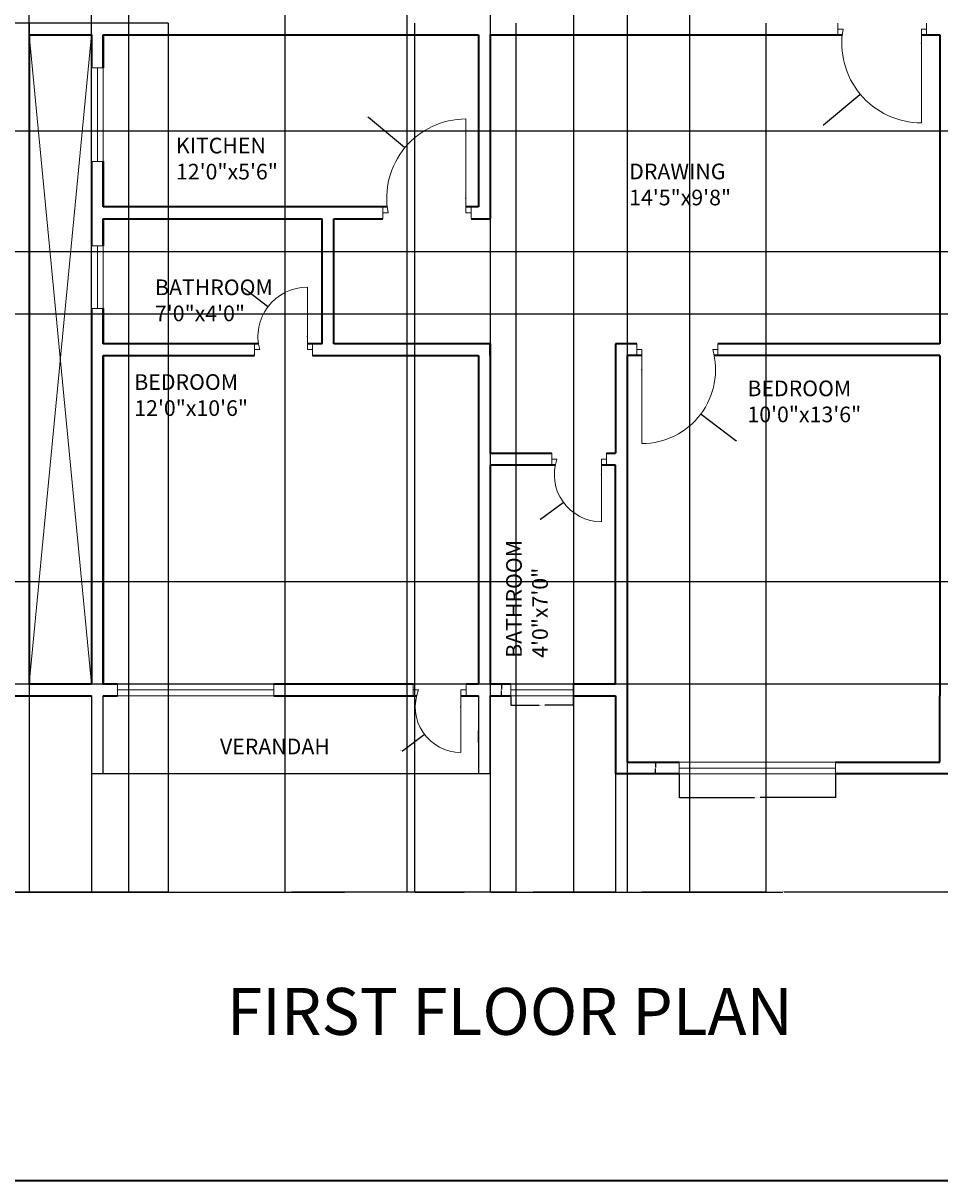
# Model space of a CAD drawing. Units: inches. Extents: x 1831 to 2867, y 1605 to 2524.
# Tile 2 of 7: x 2170 to 2522, y 1605 to 2049. Entities that reach past the tile are written whole.
import ezdxf

# ---------------------------------------------------------------- set-up
doc = ezdxf.new("R2010")
doc.units = ezdxf.units.IN
for name, color, linetype, lineweight in [('A-ANNO-DIMS', 2, 'Continuous', 18), ('A-ANNO-TEXT', 7, 'Continuous', 35), ('A-ANNO-TTLB', 7, 'Continuous', 35), ('A-AREA-IDEN', 7, 'Continuous', 18), ('A-DOOR', 11, 'Continuous', 18), ('A-FLOR-BALC', 7, 'Continuous', 25), ('A-FLOR-OPEN', 7, 'Continuous', 13), ('A-GLAZ', 121, 'Continuous', 18), ('A-WALL', 7, 'Continuous', 35)]:
    doc.layers.add(name, color=color, linetype=linetype, lineweight=lineweight)
doc.styles.get("Standard").update_dxf_attribs({"font": 'arial.ttf'})
doc.dimstyles.get("Standard").update_dxf_attribs({"dimtxt": 0.18, "dimasz": 0.18, "dimexe": 0.18, "dimexo": 0.0625, "dimgap": 0.09, "dimtad": 0, "dimtih": 1, "dimtoh": 1, "dimdec": 4, "dimzin": 0, "dimdsep": 46, "dimtxsty": 'Standard', "dimcen": 0.09, "dimadec": 0, "dimazin": 0, "dimtfac": 1, "dimtdec": 4, "dimtofl": 0, "dimtmove": 0, "dimatfit": 3, "dimfxl": 1, "dimtolj": 1, "dimtzin": 0, "dimarcsym": 0})

# ---------------------------------------------------------------- blocks, each defined once
blk = doc.blocks.new('WIN-60IN')
for p, q in [((4.5, 60), (0, 60)), ((0, 60), (2.25, 60)), ((0, 0), (0, 60)), ((2.25, 60), (2.25, 0)), ((4.5, 60), (4.5, 0)), ((4.5, 0), (0, 0)), ((2.25, 0), (4.5, 0))]:
    blk.add_line(p, q)
blk = doc.blocks.new('WIN-24IN')
for p, q in [((4.5, 24), (0, 24)), ((0, 24), (2.25, 24)), ((0, 0), (0, 24)), ((2.25, 24), (2.25, 0)), ((4.5, 0), (4.5, 24)), ((4.5, 0), (0, 0)), ((2.25, 0), (4.5, 0))]:
    blk.add_line(p, q)
blk = doc.blocks.new('WIN-36IN')
for p, q in [((0, 0), (0, 4.5)), ((36, 4.5), (0, 4.5)), ((36, 0), (36, 4.5)), ((36, 4.5), (36, 2.25)), ((36, 2.25), (0, 2.25)), ((0, 2.25), (0, 0)), ((0, 0), (36, 0))]:
    blk.add_line(p, q)
blk = doc.blocks.new('DOOR-LEAF-36IN')
for p, q in [((0, 2), (4.5, 2)), ((4.5, 2), (2.25, 2)), ((2.25, 2), (2.25, 0)), ((2.25, 0), (38.25, 0))]:
    blk.add_line(p, q)
blk = doc.blocks.new('DOOR-LEAF-36IN-ALT')
for p, q in [((36, 2), (0, 2)), ((33.75, 0), (38.25, 0)), ((36, 0), (36, 2)), ((38.25, 0), (36, 0))]:
    blk.add_line(p, q)
blk = doc.blocks.new('DOOR-LEAF-24IN')
for p, q in [((2.25, 0), (2.25, 2)), ((2.25, 2), (26.25, 2)), ((0, 0), (4.5, 0)), ((4.5, 0), (2.25, 0))]:
    blk.add_line(p, q)
blk = doc.blocks.new('DOOR-LEAF-24IN-ALT')
for p, q in [((24, 2), (0, 2)), ((21.75, 0), (26.25, 0)), ((24, 0), (24, 2)), ((26.25, 0), (24, 0))]:
    blk.add_line(p, q)
blk = doc.blocks.new('DOOR-STRIKE-JAMB')
for p, q in [((0, 0), (4.5, 0)), ((2.25, 0), (2.25, 2)), ((4.5, 0), (2.25, 0))]:
    blk.add_line(p, q)
blk = doc.blocks.new('*D16')
at = {"layer": 'A-ANNO-DIMS', "color": 0, "lineweight": -2, "transparency": 16777216}
for p, q in [((2356.89, 1791.11), (2356.89, 1787.39)), ((2380.89, 1791.11), (2380.89, 1787.39)), ((2357.07, 1787.57), (2367.77, 1787.57)), ((2380.71, 1787.57), (2370.01, 1787.57))]:
    blk.add_line(p, q, dxfattribs=at)
at = {"layer": 'A-ANNO-DIMS', "color": 0, "transparency": 16777216}
for points in [[(2357.07, 1787.6), (2357.07, 1787.54), (2356.89, 1787.57)], [(2380.71, 1787.6), (2380.71, 1787.54), (2380.89, 1787.57)]]:
    blk.add_solid(points, dxfattribs=at)
at = {"layer": 'Defpoints', "color": 0, "transparency": 16777216}
for p in [(2356.89, 1791.17), (2380.89, 1791.17), (2356.89, 1787.57)]:
    blk.add_point(p, dxfattribs=at)
at = {"layer": 'A-ANNO-DIMS', "color": 0, "transparency": 16777216, "insert": (2368.89, 1787.57), "char_height": 0.18, "attachment_point": 5}
blk.add_mtext('\\A1;WINDOW 24 TYP.', dxfattribs=at)
blk = doc.blocks.new('*D17')
at = {"layer": 'A-ANNO-DIMS', "color": 0, "lineweight": -2, "transparency": 16777216}
for p, q in [((2356.83, 1795.67), (2353.11, 1795.67)), ((2353.29, 1795.49), (2353.29, 1793.61)), ((2356.83, 1791.17), (2353.11, 1791.17)), ((2353.29, 1791.35), (2353.29, 1793.24))]:
    blk.add_line(p, q, dxfattribs=at)
at = {"layer": 'A-ANNO-DIMS', "color": 0, "transparency": 16777216}
for points in [[(2353.26, 1795.49), (2353.32, 1795.49), (2353.29, 1795.67)], [(2353.26, 1791.35), (2353.32, 1791.35), (2353.29, 1791.17)]]:
    blk.add_solid(points, dxfattribs=at)
at = {"layer": 'Defpoints', "color": 0, "transparency": 16777216}
for p in [(2353.29, 1795.67), (2356.89, 1795.67), (2356.89, 1791.17)]:
    blk.add_point(p, dxfattribs=at)
at = {"layer": 'A-ANNO-DIMS', "color": 0, "transparency": 16777216, "insert": (2353.29, 1793.42), "char_height": 0.18, "attachment_point": 5}
blk.add_mtext('\\A1;5 TYP.', dxfattribs=at)
blk = doc.blocks.new('*D20')
at = {"layer": 'A-ANNO-DIMS', "color": 0, "lineweight": -2, "transparency": 16777216}
for p, q in [((2421.49, 1761.11), (2421.49, 1751.99)), ((2481.49, 1761.11), (2481.49, 1751.99)), ((2421.67, 1752.17), (2450.37, 1752.17)), ((2481.31, 1752.17), (2452.61, 1752.17))]:
    blk.add_line(p, q, dxfattribs=at)
at = {"layer": 'A-ANNO-DIMS', "color": 0, "transparency": 16777216}
for points in [[(2421.67, 1752.2), (2421.67, 1752.14), (2421.49, 1752.17)], [(2481.31, 1752.2), (2481.31, 1752.14), (2481.49, 1752.17)]]:
    blk.add_solid(points, dxfattribs=at)
at = {"layer": 'Defpoints', "color": 0, "transparency": 16777216}
for p in [(2421.49, 1761.17), (2481.49, 1761.17), (2421.49, 1752.17)]:
    blk.add_point(p, dxfattribs=at)
at = {"layer": 'A-ANNO-DIMS', "color": 0, "transparency": 16777216, "insert": (2451.49, 1752.17), "char_height": 0.18, "attachment_point": 5}
blk.add_mtext('\\A1;WINDOW 60 TYP.', dxfattribs=at)
blk = doc.blocks.new('*D21')
at = {"layer": 'A-ANNO-DIMS', "color": 0, "lineweight": -2, "transparency": 16777216}
for p, q in [((2421.43, 1765.67), (2412.31, 1765.67)), ((2412.49, 1765.49), (2412.49, 1763.61)), ((2412.49, 1761.35), (2412.49, 1763.24)), ((2421.43, 1761.17), (2412.31, 1761.17))]:
    blk.add_line(p, q, dxfattribs=at)
at = {"layer": 'A-ANNO-DIMS', "color": 0, "transparency": 16777216}
for points in [[(2412.46, 1765.49), (2412.52, 1765.49), (2412.49, 1765.67)], [(2412.46, 1761.35), (2412.52, 1761.35), (2412.49, 1761.17)]]:
    blk.add_solid(points, dxfattribs=at)
at = {"layer": 'Defpoints', "color": 0, "transparency": 16777216}
for p in [(2412.49, 1765.67), (2421.49, 1765.67), (2421.49, 1761.17)]:
    blk.add_point(p, dxfattribs=at)
at = {"layer": 'A-ANNO-DIMS', "color": 0, "transparency": 16777216, "insert": (2412.49, 1763.42), "char_height": 0.18, "attachment_point": 5}
blk.add_mtext('\\A1;5 TYP.', dxfattribs=at)
blk = doc.blocks.new('*D25')
at = {"layer": 'A-ANNO-DIMS', "color": 0, "lineweight": -2, "transparency": 16777216}
for p, q in [((2055.05, 1761.11), (2055.05, 1715.69)), ((2196.05, 1761.11), (2196.05, 1715.69)), ((2055.23, 1715.87), (2125.29, 1715.87)), ((2195.87, 1715.87), (2125.81, 1715.87))]:
    blk.add_line(p, q, dxfattribs=at)
at = {"layer": 'A-ANNO-DIMS', "color": 0, "transparency": 16777216}
for points in [[(2055.23, 1715.9), (2055.23, 1715.84), (2055.05, 1715.87)], [(2195.87, 1715.9), (2195.87, 1715.84), (2196.05, 1715.87)]]:
    blk.add_solid(points, dxfattribs=at)
at = {"layer": 'Defpoints', "color": 0, "transparency": 16777216}
for p in [(2055.05, 1761.17), (2196.05, 1761.17), (2196.05, 1715.87)]:
    blk.add_point(p, dxfattribs=at)
at = {"layer": 'A-ANNO-DIMS', "color": 0, "transparency": 16777216, "insert": (2125.55, 1715.87), "char_height": 0.18, "attachment_point": 5}
blk.add_mtext('\\A1;141', dxfattribs=at)
blk = doc.blocks.new('*D26')
at = {"layer": 'A-ANNO-DIMS', "color": 0, "lineweight": -2, "transparency": 16777216}
for p, q in [((2196.05, 1761.11), (2196.05, 1715.69)), ((2349.05, 1761.11), (2349.05, 1715.69)), ((2196.23, 1715.87), (2272.27, 1715.87)), ((2348.87, 1715.87), (2272.83, 1715.87))]:
    blk.add_line(p, q, dxfattribs=at)
at = {"layer": 'A-ANNO-DIMS', "color": 0, "transparency": 16777216}
for points in [[(2196.23, 1715.9), (2196.23, 1715.84), (2196.05, 1715.87)], [(2348.87, 1715.9), (2348.87, 1715.84), (2349.05, 1715.87)]]:
    blk.add_solid(points, dxfattribs=at)
at = {"layer": 'Defpoints', "color": 0, "transparency": 16777216}
for p in [(2196.05, 1761.17), (2349.05, 1761.17), (2349.05, 1715.87)]:
    blk.add_point(p, dxfattribs=at)
at = {"layer": 'A-ANNO-DIMS', "color": 0, "transparency": 16777216, "insert": (2272.55, 1715.87), "char_height": 0.18, "attachment_point": 5}
blk.add_mtext('\\A1;153', dxfattribs=at)
blk = doc.blocks.new('*D27')
at = {"layer": 'A-ANNO-DIMS', "color": 0, "lineweight": -2, "transparency": 16777216}
for p, q in [((2349.05, 1761.11), (2349.05, 1715.69)), ((2397.05, 1761.11), (2397.05, 1715.69)), ((2349.23, 1715.87), (2372.83, 1715.87)), ((2396.87, 1715.87), (2373.27, 1715.87))]:
    blk.add_line(p, q, dxfattribs=at)
at = {"layer": 'A-ANNO-DIMS', "color": 0, "transparency": 16777216}
for points in [[(2349.23, 1715.9), (2349.23, 1715.84), (2349.05, 1715.87)], [(2396.87, 1715.9), (2396.87, 1715.84), (2397.05, 1715.87)]]:
    blk.add_solid(points, dxfattribs=at)
at = {"layer": 'Defpoints', "color": 0, "transparency": 16777216}
for p in [(2349.05, 1761.17), (2397.05, 1761.17), (2397.05, 1715.87)]:
    blk.add_point(p, dxfattribs=at)
at = {"layer": 'A-ANNO-DIMS', "color": 0, "transparency": 16777216, "insert": (2373.05, 1715.87), "char_height": 0.18, "attachment_point": 5}
blk.add_mtext('\\A1;48', dxfattribs=at)
blk = doc.blocks.new('*D28')
at = {"layer": 'A-ANNO-DIMS', "color": 0, "lineweight": -2, "transparency": 16777216}
for p, q in [((2397.05, 1761.11), (2397.05, 1715.69)), ((2526.05, 1761.11), (2526.05, 1715.69)), ((2397.23, 1715.87), (2461.27, 1715.87)), ((2525.87, 1715.87), (2461.83, 1715.87))]:
    blk.add_line(p, q, dxfattribs=at)
at = {"layer": 'A-ANNO-DIMS', "color": 0, "transparency": 16777216}
for points in [[(2397.23, 1715.9), (2397.23, 1715.84), (2397.05, 1715.87)], [(2525.87, 1715.9), (2525.87, 1715.84), (2526.05, 1715.87)]]:
    blk.add_solid(points, dxfattribs=at)
at = {"layer": 'Defpoints', "color": 0, "transparency": 16777216}
for p in [(2397.05, 1761.17), (2526.05, 1761.17), (2526.05, 1715.87)]:
    blk.add_point(p, dxfattribs=at)
at = {"layer": 'A-ANNO-DIMS', "color": 0, "transparency": 16777216, "insert": (2461.55, 1715.87), "char_height": 0.18, "attachment_point": 5}
blk.add_mtext('\\A1;129', dxfattribs=at)
blk = doc.blocks.new('*D41')
at = {"layer": 'A-ANNO-DIMS', "color": 0, "lineweight": -2, "transparency": 16777216}
for p, q in [((2156.64, 2387.11), (2156.64, 1715.69)), ((2210.17, 2387.11), (2210.17, 1715.69)), ((2156.82, 1715.87), (2183.01, 1715.87)), ((2209.99, 1715.87), (2183.8, 1715.87))]:
    blk.add_line(p, q, dxfattribs=at)
at = {"layer": 'A-ANNO-DIMS', "color": 0, "transparency": 16777216}
for points in [[(2156.82, 1715.9), (2156.82, 1715.84), (2156.64, 1715.87)], [(2209.99, 1715.9), (2209.99, 1715.84), (2210.17, 1715.87)]]:
    blk.add_solid(points, dxfattribs=at)
at = {"layer": 'Defpoints', "color": 0, "transparency": 16777216}
for p in [(2156.64, 2387.17), (2210.17, 2387.17), (2210.17, 1715.87)]:
    blk.add_point(p, dxfattribs=at)
at = {"layer": 'A-ANNO-DIMS', "color": 0, "transparency": 16777216, "insert": (2183.4, 1715.87), "char_height": 0.18, "attachment_point": 5}
blk.add_mtext('\\A1;53.52', dxfattribs=at)
blk = doc.blocks.new('*D42')
at = {"layer": 'A-ANNO-DIMS', "color": 0, "lineweight": -2, "transparency": 16777216}
for p, q in [((2270.17, 2391.61), (2270.17, 1715.69)), ((2316.97, 2391.61), (2316.97, 1715.69)), ((2270.35, 1715.87), (2293.1, 1715.87)), ((2316.79, 1715.87), (2294.04, 1715.87))]:
    blk.add_line(p, q, dxfattribs=at)
at = {"layer": 'A-ANNO-DIMS', "color": 0, "transparency": 16777216}
for points in [[(2270.35, 1715.9), (2270.35, 1715.84), (2270.17, 1715.87)], [(2316.79, 1715.9), (2316.79, 1715.84), (2316.97, 1715.87)]]:
    blk.add_solid(points, dxfattribs=at)
at = {"layer": 'Defpoints', "color": 0, "transparency": 16777216}
for p in [(2270.17, 2391.67), (2316.97, 2391.67), (2316.97, 1715.87)]:
    blk.add_point(p, dxfattribs=at)
at = {"layer": 'A-ANNO-DIMS', "color": 0, "transparency": 16777216, "insert": (2293.57, 1715.87), "char_height": 0.18, "attachment_point": 5}
blk.add_mtext('\\A1;46.805', dxfattribs=at)
blk = doc.blocks.new('*D43')
at = {"layer": 'A-ANNO-DIMS', "color": 0, "lineweight": -2, "transparency": 16777216}
for p, q in [((2349.05, 2387.11), (2349.05, 1715.69)), ((2381.01, 2387.11), (2381.01, 1715.69)), ((2349.23, 1715.87), (2364.57, 1715.87)), ((2380.83, 1715.87), (2365.49, 1715.87))]:
    blk.add_line(p, q, dxfattribs=at)
at = {"layer": 'A-ANNO-DIMS', "color": 0, "transparency": 16777216}
for points in [[(2349.23, 1715.9), (2349.23, 1715.84), (2349.05, 1715.87)], [(2380.83, 1715.9), (2380.83, 1715.84), (2381.01, 1715.87)]]:
    blk.add_solid(points, dxfattribs=at)
at = {"layer": 'Defpoints', "color": 0, "transparency": 16777216}
for p in [(2349.05, 2387.17), (2381.01, 2387.17), (2381.01, 1715.87)]:
    blk.add_point(p, dxfattribs=at)
at = {"layer": 'A-ANNO-DIMS', "color": 0, "transparency": 16777216, "insert": (2365.03, 1715.87), "char_height": 0.18, "attachment_point": 5}
blk.add_mtext('\\A1;31.956', dxfattribs=at)
blk = doc.blocks.new('*D44')
at = {"layer": 'A-ANNO-DIMS', "color": 0, "lineweight": -2, "transparency": 16777216}
for p, q in [((2401.55, 2417.11), (2401.55, 1715.69)), ((2425.47, 2417.11), (2425.47, 1715.69)), ((2401.73, 1715.87), (2413.05, 1715.87)), ((2425.29, 1715.87), (2413.98, 1715.87))]:
    blk.add_line(p, q, dxfattribs=at)
at = {"layer": 'A-ANNO-DIMS', "color": 0, "transparency": 16777216}
for points in [[(2401.73, 1715.9), (2401.73, 1715.84), (2401.55, 1715.87)], [(2425.29, 1715.9), (2425.29, 1715.84), (2425.47, 1715.87)]]:
    blk.add_solid(points, dxfattribs=at)
at = {"layer": 'Defpoints', "color": 0, "transparency": 16777216}
for p in [(2401.55, 2417.17), (2425.47, 2417.17), (2425.47, 1715.87)]:
    blk.add_point(p, dxfattribs=at)
at = {"layer": 'A-ANNO-DIMS', "color": 0, "transparency": 16777216, "insert": (2413.51, 1715.87), "char_height": 0.18, "attachment_point": 5}
blk.add_mtext('\\A1;23.924', dxfattribs=at)
blk = doc.blocks.new('*D53')
at = {"layer": 'A-ANNO-DIMS', "color": 0, "lineweight": -2, "transparency": 16777216}
for p, q in [((2786.99, 2007.7), (1844.57, 2007.7)), ((1844.75, 2007.52), (1844.75, 1984.78)), ((1844.75, 1961.67), (1844.75, 1984.41)), ((2786.99, 1961.49), (1844.57, 1961.49))]:
    blk.add_line(p, q, dxfattribs=at)
at = {"layer": 'A-ANNO-DIMS', "color": 0, "transparency": 16777216}
for points in [[(1844.72, 2007.52), (1844.78, 2007.52), (1844.75, 2007.7)], [(1844.72, 1961.67), (1844.78, 1961.67), (1844.75, 1961.49)]]:
    blk.add_solid(points, dxfattribs=at)
at = {"layer": 'Defpoints', "color": 0, "transparency": 16777216}
for p in [(2787.05, 2007.7), (1844.75, 1961.49), (2787.05, 1961.49)]:
    blk.add_point(p, dxfattribs=at)
at = {"layer": 'A-ANNO-DIMS', "color": 0, "transparency": 16777216, "insert": (1844.75, 1984.59), "char_height": 0.18, "attachment_point": 5}
blk.add_mtext('\\A1;46.2', dxfattribs=at)
blk = doc.blocks.new('*D54')
at = {"layer": 'A-ANNO-DIMS', "color": 0, "lineweight": -2, "transparency": 16777216}
for p, q in [((2786.99, 1937.49), (1844.57, 1937.49)), ((1844.75, 1937.31), (1844.75, 1886.37)), ((1844.75, 1835.06), (1844.75, 1886)), ((2786.99, 1834.88), (1844.57, 1834.88))]:
    blk.add_line(p, q, dxfattribs=at)
at = {"layer": 'A-ANNO-DIMS', "color": 0, "transparency": 16777216}
for points in [[(1844.72, 1937.31), (1844.78, 1937.31), (1844.75, 1937.49)], [(1844.72, 1835.06), (1844.78, 1835.06), (1844.75, 1834.88)]]:
    blk.add_solid(points, dxfattribs=at)
at = {"layer": 'Defpoints', "color": 0, "transparency": 16777216}
for p in [(2787.05, 1937.49), (1844.75, 1834.88), (2787.05, 1834.88)]:
    blk.add_point(p, dxfattribs=at)
at = {"layer": 'A-ANNO-DIMS', "color": 0, "transparency": 16777216, "insert": (1844.75, 1886.19), "char_height": 0.18, "attachment_point": 5}
blk.add_mtext('\\A1;102.61', dxfattribs=at)
blk = doc.blocks.new('*D55')
at = {"layer": 'A-ANNO-DIMS', "color": 0, "lineweight": -2, "transparency": 16777216}
for p, q in [((2786.99, 1834.88), (1844.57, 1834.88)), ((1844.75, 1834.7), (1844.75, 1815.46)), ((1844.75, 1795.85), (1844.75, 1815.09)), ((2786.99, 1795.67), (1844.57, 1795.67))]:
    blk.add_line(p, q, dxfattribs=at)
at = {"layer": 'A-ANNO-DIMS', "color": 0, "transparency": 16777216}
for points in [[(1844.72, 1834.7), (1844.78, 1834.7), (1844.75, 1834.88)], [(1844.72, 1795.85), (1844.78, 1795.85), (1844.75, 1795.67)]]:
    blk.add_solid(points, dxfattribs=at)
at = {"layer": 'Defpoints', "color": 0, "transparency": 16777216}
for p in [(2787.05, 1834.88), (1844.75, 1795.67), (2787.05, 1795.67)]:
    blk.add_point(p, dxfattribs=at)
at = {"layer": 'A-ANNO-DIMS', "color": 0, "transparency": 16777216, "insert": (1844.75, 1815.28), "char_height": 0.18, "attachment_point": 5}
blk.add_mtext('\\A1;39.206', dxfattribs=at)
blk = doc.blocks.new('*D56')
at = {"layer": 'A-ANNO-DIMS', "color": 0, "lineweight": -2, "transparency": 16777216}
for p, q in [((2172.05, 2049.11), (2172.05, 1715.69)), ((2225.49, 2049.11), (2225.49, 1715.69)), ((2172.23, 1715.87), (2198.38, 1715.87)), ((2225.31, 1715.87), (2199.17, 1715.87))]:
    blk.add_line(p, q, dxfattribs=at)
at = {"layer": 'A-ANNO-DIMS', "color": 0, "transparency": 16777216}
for points in [[(2172.23, 1715.9), (2172.23, 1715.84), (2172.05, 1715.87)], [(2225.31, 1715.9), (2225.31, 1715.84), (2225.49, 1715.87)]]:
    blk.add_solid(points, dxfattribs=at)
at = {"layer": 'Defpoints', "color": 0, "transparency": 16777216}
for p in [(2172.05, 2049.17), (2225.49, 2049.17), (2225.49, 1715.87)]:
    blk.add_point(p, dxfattribs=at)
at = {"layer": 'A-ANNO-DIMS', "color": 0, "transparency": 16777216, "insert": (2198.77, 1715.87), "char_height": 0.18, "attachment_point": 5}
blk.add_mtext('\\A1;53.44', dxfattribs=at)
blk = doc.blocks.new('*D57')
at = {"layer": 'A-ANNO-DIMS', "color": 0, "lineweight": -2, "transparency": 16777216}
for p, q in [((2225.49, 2049.11), (2225.49, 1715.69)), ((2319.99, 2049.11), (2319.99, 1715.69)), ((2225.67, 1715.87), (2272.42, 1715.87)), ((2319.81, 1715.87), (2273.06, 1715.87))]:
    blk.add_line(p, q, dxfattribs=at)
at = {"layer": 'A-ANNO-DIMS', "color": 0, "transparency": 16777216}
for points in [[(2225.67, 1715.9), (2225.67, 1715.84), (2225.49, 1715.87)], [(2319.81, 1715.9), (2319.81, 1715.84), (2319.99, 1715.87)]]:
    blk.add_solid(points, dxfattribs=at)
at = {"layer": 'Defpoints', "color": 0, "transparency": 16777216}
for p in [(2225.49, 2049.17), (2319.99, 2049.17), (2319.99, 1715.87)]:
    blk.add_point(p, dxfattribs=at)
at = {"layer": 'A-ANNO-DIMS', "color": 0, "transparency": 16777216, "insert": (2272.74, 1715.87), "char_height": 0.18, "attachment_point": 5}
blk.add_mtext('\\A1;94.5', dxfattribs=at)
blk = doc.blocks.new('*D58')
at = {"layer": 'A-ANNO-DIMS', "color": 0, "lineweight": -2, "transparency": 16777216}
for p, q in [((2319.99, 2049.11), (2319.99, 1715.69)), ((2358.81, 2049.11), (2358.81, 1715.69)), ((2320.17, 1715.87), (2339, 1715.87)), ((2358.63, 1715.87), (2339.79, 1715.87))]:
    blk.add_line(p, q, dxfattribs=at)
at = {"layer": 'A-ANNO-DIMS', "color": 0, "transparency": 16777216}
for points in [[(2320.17, 1715.9), (2320.17, 1715.84), (2319.99, 1715.87)], [(2358.63, 1715.9), (2358.63, 1715.84), (2358.81, 1715.87)]]:
    blk.add_solid(points, dxfattribs=at)
at = {"layer": 'Defpoints', "color": 0, "transparency": 16777216}
for p in [(2319.99, 2049.17), (2358.81, 2049.17), (2358.81, 1715.87)]:
    blk.add_point(p, dxfattribs=at)
at = {"layer": 'A-ANNO-DIMS', "color": 0, "transparency": 16777216, "insert": (2339.4, 1715.87), "char_height": 0.18, "attachment_point": 5}
blk.add_mtext('\\A1;38.82', dxfattribs=at)
blk = doc.blocks.new('*D59')
at = {"layer": 'A-ANNO-DIMS', "color": 0, "lineweight": -2, "transparency": 16777216}
for p, q in [((2358.81, 2049.11), (2358.81, 1715.69)), ((2454.81, 2049.11), (2454.81, 1715.69)), ((2358.99, 1715.87), (2406.59, 1715.87)), ((2454.63, 1715.87), (2407.02, 1715.87))]:
    blk.add_line(p, q, dxfattribs=at)
at = {"layer": 'A-ANNO-DIMS', "color": 0, "transparency": 16777216}
for points in [[(2358.99, 1715.9), (2358.99, 1715.84), (2358.81, 1715.87)], [(2454.63, 1715.9), (2454.63, 1715.84), (2454.81, 1715.87)]]:
    blk.add_solid(points, dxfattribs=at)
at = {"layer": 'Defpoints', "color": 0, "transparency": 16777216}
for p in [(2358.81, 2049.17), (2454.81, 2049.17), (2454.81, 1715.87)]:
    blk.add_point(p, dxfattribs=at)
at = {"layer": 'A-ANNO-DIMS', "color": 0, "transparency": 16777216, "insert": (2406.81, 1715.87), "char_height": 0.18, "attachment_point": 5}
blk.add_mtext('\\A1;96', dxfattribs=at)
blk = doc.blocks.new('*D60')
at = {"layer": 'A-ANNO-DIMS', "color": 0, "lineweight": -2, "transparency": 16777216}
for p, q in [((2225.43, 2091.42), (1844.57, 2091.42)), ((1844.75, 2091.24), (1844.75, 2070.48)), ((1844.75, 2049.35), (1844.75, 2070.12)), ((2225.43, 2049.17), (1844.57, 2049.17))]:
    blk.add_line(p, q, dxfattribs=at)
at = {"layer": 'A-ANNO-DIMS', "color": 0, "transparency": 16777216}
for points in [[(1844.72, 2091.24), (1844.78, 2091.24), (1844.75, 2091.42)], [(1844.72, 2049.35), (1844.78, 2049.35), (1844.75, 2049.17)]]:
    blk.add_solid(points, dxfattribs=at)
at = {"layer": 'Defpoints', "color": 0, "transparency": 16777216}
for p in [(1844.75, 2091.42), (2225.49, 2091.42), (2225.49, 2049.17)]:
    blk.add_point(p, dxfattribs=at)
at = {"layer": 'A-ANNO-DIMS', "color": 0, "transparency": 16777216, "insert": (1844.75, 2070.3), "char_height": 0.18, "attachment_point": 5}
blk.add_mtext('\\A1;42.25', dxfattribs=at)
blk = doc.blocks.new('*D63')
at = {"layer": 'A-ANNO-DIMS', "color": 0, "lineweight": -2, "transparency": 16777216}
for p, q in [((2172.05, 1795.74), (2172.05, 2467.15)), ((2172.23, 2466.97), (2183.83, 2466.97)), ((2195.87, 2466.97), (2184.27, 2466.97)), ((2196.05, 1795.74), (2196.05, 2467.15))]:
    blk.add_line(p, q, dxfattribs=at)
at = {"layer": 'A-ANNO-DIMS', "color": 0, "transparency": 16777216}
for points in [[(2172.23, 2467), (2172.23, 2466.94), (2172.05, 2466.97)], [(2195.87, 2467), (2195.87, 2466.94), (2196.05, 2466.97)]]:
    blk.add_solid(points, dxfattribs=at)
at = {"layer": 'Defpoints', "color": 0, "transparency": 16777216}
for p in [(2196.05, 2466.97), (2172.05, 1795.67), (2196.05, 1795.67)]:
    blk.add_point(p, dxfattribs=at)
at = {"layer": 'A-ANNO-DIMS', "color": 0, "transparency": 16777216, "insert": (2184.05, 2466.97), "char_height": 0.18, "attachment_point": 5}
blk.add_mtext('\\A1;24', dxfattribs=at)
blk = doc.blocks.new('*D66')
at = {"layer": 'A-ANNO-DIMS', "color": 0, "lineweight": -2, "transparency": 16777216}
for p, q in [((2514.4, 2041.48), (2514.58, 2041.48)), ((2514.49, 2041.39), (2514.49, 2041.57)), ((2476.96, 2010.14), (2490.9, 2021.78)), ((2476.78, 2010.14), (2476.96, 2010.14))]:
    blk.add_line(p, q, dxfattribs=at)
at = {"layer": 'A-ANNO-DIMS', "color": 0, "transparency": 16777216}
blk.add_solid([(2490.88, 2021.8), (2490.92, 2021.75), (2491.04, 2021.89)], dxfattribs=at)
at = {"layer": 'Defpoints', "color": 0, "transparency": 16777216}
for p in [(2514.49, 2041.48), (2491.04, 2021.89)]:
    blk.add_point(p, dxfattribs=at)
at = {"layer": 'A-ANNO-DIMS', "color": 0, "transparency": 16777216, "insert": (2476.3, 2010.14), "char_height": 0.18, "attachment_point": 5}
blk.add_mtext('\\A1;R30.56', dxfattribs=at)
blk = doc.blocks.new('*D67')
at = {"layer": 'A-ANNO-DIMS', "color": 0, "lineweight": -2, "transparency": 16777216}
for p, q in [((2302.1, 2013.08), (2302.28, 2013.08)), ((2302.28, 2013.08), (2316.18, 2001.55)), ((2339.62, 1982.03), (2339.8, 1982.03)), ((2339.71, 1981.94), (2339.71, 1982.12))]:
    blk.add_line(p, q, dxfattribs=at)
at = {"layer": 'A-ANNO-DIMS', "color": 0, "transparency": 16777216}
blk.add_solid([(2316.2, 2001.58), (2316.16, 2001.53), (2316.32, 2001.44)], dxfattribs=at)
at = {"layer": 'Defpoints', "color": 0, "transparency": 16777216}
for p in [(2316.32, 2001.44), (2339.71, 1982.03)]:
    blk.add_point(p, dxfattribs=at)
at = {"layer": 'A-ANNO-DIMS', "color": 0, "transparency": 16777216, "insert": (2301.55, 2013.08), "char_height": 0.18, "attachment_point": 5}
blk.add_mtext('\\A1;R30.395', dxfattribs=at)
blk = doc.blocks.new('*D71')
at = {"layer": 'A-ANNO-DIMS', "color": 0, "lineweight": -2, "transparency": 16777216}
for p, q in [((2407.14, 1916.17), (2407.32, 1916.17)), ((2407.23, 1916.08), (2407.23, 1916.26)), ((2443.31, 1888.95), (2429.92, 1899.05)), ((2443.49, 1888.95), (2443.31, 1888.95))]:
    blk.add_line(p, q, dxfattribs=at)
at = {"layer": 'A-ANNO-DIMS', "color": 0, "transparency": 16777216}
blk.add_solid([(2429.94, 1899.07), (2429.9, 1899.03), (2429.78, 1899.16)], dxfattribs=at)
at = {"layer": 'Defpoints', "color": 0, "transparency": 16777216}
for p in [(2407.23, 1916.17), (2429.78, 1899.16)]:
    blk.add_point(p, dxfattribs=at)
at = {"layer": 'A-ANNO-DIMS', "color": 0, "transparency": 16777216, "insert": (2443.97, 1888.95), "char_height": 0.18, "attachment_point": 5}
blk.add_mtext('\\A1;R28.25', dxfattribs=at)
blk = doc.blocks.new('*D90')
at = {"layer": 'A-ANNO-DIMS', "color": 0, "lineweight": -2, "transparency": 16777216}
for p, q in [((2254.54, 1947.34), (2254.72, 1947.34)), ((2254.72, 1947.34), (2263.62, 1940.56)), ((2278.76, 1928.97), (2278.94, 1928.97)), ((2278.85, 1928.88), (2278.85, 1929.06))]:
    blk.add_line(p, q, dxfattribs=at)
at = {"layer": 'A-ANNO-DIMS', "color": 0, "transparency": 16777216}
blk.add_solid([(2263.64, 1940.58), (2263.61, 1940.54), (2263.77, 1940.45)], dxfattribs=at)
at = {"layer": 'Defpoints', "color": 0, "transparency": 16777216}
for p in [(2263.77, 1940.45), (2278.85, 1928.97)]:
    blk.add_point(p, dxfattribs=at)
at = {"layer": 'A-ANNO-DIMS', "color": 0, "transparency": 16777216, "insert": (2253.99, 1947.34), "char_height": 0.18, "attachment_point": 5}
blk.add_mtext('\\A1;R18.956', dxfattribs=at)
blk = doc.blocks.new('*D98')
at = {"layer": 'A-ANNO-DIMS', "color": 0, "lineweight": -2, "transparency": 16777216}
for p, q in [((2391.61, 1876), (2391.79, 1876)), ((2391.7, 1875.91), (2391.7, 1876.09)), ((2368.34, 1858.95), (2376.95, 1865.24)), ((2368.16, 1858.95), (2368.34, 1858.95))]:
    blk.add_line(p, q, dxfattribs=at)
at = {"layer": 'A-ANNO-DIMS', "color": 0, "transparency": 16777216}
blk.add_solid([(2376.93, 1865.26), (2376.97, 1865.21), (2377.1, 1865.34)], dxfattribs=at)
at = {"layer": 'Defpoints', "color": 0, "transparency": 16777216}
for p in [(2391.7, 1876), (2377.1, 1865.34)]:
    blk.add_point(p, dxfattribs=at)
at = {"layer": 'A-ANNO-DIMS', "color": 0, "transparency": 16777216, "insert": (2367.61, 1858.95), "char_height": 0.18, "attachment_point": 5}
blk.add_mtext('\\A1;R18.077', dxfattribs=at)
blk = doc.blocks.new('*D101')
at = {"layer": 'A-ANNO-DIMS', "color": 0, "lineweight": -2, "transparency": 16777216}
for p, q in [((2337.64, 1786.9), (2337.82, 1786.9)), ((2337.73, 1786.81), (2337.73, 1786.99)), ((2315.4, 1770.07), (2323.63, 1776.27)), ((2315.22, 1770.07), (2315.4, 1770.07))]:
    blk.add_line(p, q, dxfattribs=at)
at = {"layer": 'A-ANNO-DIMS', "color": 0, "transparency": 16777216}
blk.add_solid([(2323.61, 1776.3), (2323.65, 1776.25), (2323.77, 1776.38)], dxfattribs=at)
at = {"layer": 'Defpoints', "color": 0, "transparency": 16777216}
for p in [(2337.73, 1786.9), (2323.77, 1776.38)]:
    blk.add_point(p, dxfattribs=at)
at = {"layer": 'A-ANNO-DIMS', "color": 0, "transparency": 16777216, "insert": (2314.74, 1770.07), "char_height": 0.18, "attachment_point": 5}
blk.add_mtext('\\A1;R17.48', dxfattribs=at)

msp = doc.modelspace()

# ---------------------------------------------------------------- linework, layer by layer
at = {"layer": 'A-ANNO-TTLB'}
msp.add_lwpolyline([(1831.1248, 2523.9204), (2867.0416, 2523.9204), (2867.0416, 1605.0781), (1831.1248, 1605.0781)], close=True, dxfattribs=at)
at = {"layer": 'A-DOOR'}
for centre, radius, start, end in [((2514.4879, 2041.481), 30.5572, 169.739837, 270), ((2339.7066, 1982.0286), 30.3952, 90, 190.626041), ((2278.8502, 1928.9679), 18.9559, 90, 195.432084), ((2407.228, 1916.1727), 28.2489, 270, 15.925435), ((2391.6972, 1876.0006), 18.0768, 160.872592, 270), ((2337.7334, 1786.9033), 17.4795, 158.097162, 270)]:
    msp.add_arc(centre, radius, start, end, dxfattribs=at)
at = {"layer": 'A-FLOR-BALC'}
for p, q in [((2196.051, 1791.1738), (2196.051, 1761.1738)), ((2200.551, 1761.1738), (2200.551, 1791.1738)), ((2344.551, 1791.1738), (2344.551, 1761.1738)), ((2349.051, 1761.1738), (2349.051, 1791.1738)), ((2344.551, 1773.1738), (2344.551, 1777.6738)), ((2349.051, 1761.1738), (2196.051, 1761.1738))]:
    msp.add_line(p, q, dxfattribs=at)
at = {"layer": 'A-FLOR-OPEN'}
for p, q in [((2172.051, 1795.6738), (2196.051, 2044.6738)), ((2172.051, 2044.6738), (2196.051, 1795.6738))]:
    msp.add_line(p, q, dxfattribs=at)
at = {"layer": 'A-WALL'}
for p, q in [((2172.051, 2044.6738), (2196.051, 2044.6738)), ((2172.051, 2044.6738), (2172.051, 1795.6738)), ((2196.051, 2044.6738), (2196.051, 2032.0726)), ((2200.551, 2044.6738), (2200.551, 2032.0726)), ((2200.551, 2044.6738), (2344.551, 2044.6738)), ((2200.551, 2032.0726), (2200.551, 2044.6738)), ((2344.551, 2044.6738), (2344.551, 1978.6738)), ((2349.051, 2044.6738), (2349.051, 1974.1738)), ((2349.051, 2044.6738), (2484.098, 2044.6738)), ((2514.4879, 2044.6738), (2521.551, 2044.6738)), ((2521.551, 2044.6738), (2521.551, 1926.1738)), ((2196.051, 1996.0726), (2196.051, 1963.6917)), ((2200.551, 1978.6738), (2200.551, 1996.0726)), ((2200.551, 1996.0726), (2200.551, 1978.6738)), ((2309.4971, 1978.6738), (2200.551, 1978.6738)), ((2344.551, 1978.6738), (2339.7066, 1978.6738)), ((2200.551, 1974.1738), (2284.551, 1974.1738)), ((2200.551, 1974.1738), (2200.551, 1963.6917)), ((2200.551, 1963.6917), (2200.551, 1974.1738)), ((2284.551, 1926.1738), (2284.551, 1974.1738)), ((2289.051, 1926.1738), (2289.051, 1974.1738)), ((2289.051, 1974.1738), (2307.8327, 1974.1738)), ((2341.7066, 1974.1738), (2349.051, 1974.1738)), ((2196.051, 1939.6917), (2196.051, 1795.6738)), ((2200.551, 1926.1738), (2200.551, 1939.6917)), ((2200.551, 1939.6917), (2200.551, 1926.1738)), ((2260.1014, 1926.1738), (2200.551, 1926.1738)), ((2284.551, 1926.1738), (2278.8502, 1926.1738)), ((2349.051, 1926.1738), (2289.051, 1926.1738)), ((2349.051, 1921.6738), (2349.051, 1926.1738)), ((2349.051, 1926.1738), (2349.051, 1884.1738)), ((2397.051, 1926.1738), (2397.051, 1884.1738)), ((2405.228, 1926.1738), (2397.051, 1926.1738)), ((2521.551, 1926.1738), (2436.3927, 1926.1738)), ((2200.551, 1795.6738), (2200.551, 1921.6738)), ((2200.551, 1921.6738), (2258.5778, 1921.6738)), ((2200.551, 1921.6738), (2200.551, 1795.6738)), ((2280.8502, 1921.6738), (2344.551, 1921.6738)), ((2344.551, 1921.6738), (2344.551, 1795.6738)), ((2401.551, 1921.6738), (2401.551, 1884.1738)), ((2407.228, 1921.6738), (2401.551, 1921.6738)), ((2521.551, 1921.6738), (2434.9361, 1921.6738)), ((2521.551, 1921.6738), (2521.551, 1791.1738)), ((2349.051, 1884.1738), (2372.6184, 1884.1738)), ((2393.6972, 1884.1738), (2397.051, 1884.1738)), ((2401.551, 1884.1738), (2401.551, 1795.6738)), ((2352.727, 1879.6738), (2349.051, 1879.6738)), ((2349.051, 1879.6738), (2349.051, 1795.6738)), ((2373.9975, 1879.6738), (2352.727, 1879.6738)), ((2397.051, 1879.6738), (2391.6972, 1879.6738)), ((2397.051, 1795.6738), (2397.051, 1879.6738)), ((2172.051, 1795.6738), (2196.051, 1795.6738)), ((2200.551, 1795.6738), (2206.0469, 1795.6738)), ((2266.0469, 1795.6738), (2319.5155, 1795.6738)), ((2339.7334, 1795.6738), (2344.551, 1795.6738)), ((2349.051, 1795.6738), (2356.8929, 1795.6738)), ((2349.051, 1795.6738), (2356.8929, 1795.6738)), ((2380.8929, 1795.6738), (2397.051, 1795.6738)), ((2380.8929, 1795.6738), (2397.051, 1795.6738)), ((2401.551, 1795.6738), (2401.551, 1765.6738)), ((2161.4296, 1791.1738), (2196.051, 1791.1738)), ((2200.551, 1791.1738), (2206.0469, 1791.1738)), ((2266.0469, 1791.1738), (2320.7835, 1791.1738)), ((2337.7334, 1791.1738), (2344.551, 1791.1738)), ((2349.051, 1791.1738), (2356.8929, 1791.1738)), ((2380.8929, 1791.1738), (2397.051, 1791.1738)), ((2397.051, 1791.1738), (2397.051, 1761.1738)), ((2521.551, 1765.6738), (2521.551, 1791.1738)), ((2401.551, 1765.6738), (2421.4899, 1765.6738)), ((2481.4899, 1765.6738), (2521.551, 1765.6738)), ((2421.4899, 1761.1738), (2397.051, 1761.1738)), ((2526.051, 1761.1738), (2481.4899, 1761.1738))]:
    msp.add_line(p, q, dxfattribs=at)

# ---------------------------------------------------------------- block references
at = {"layer": 'A-DOOR'}
for name, p, rotation in [('DOOR-STRIKE-JAMB', (2482.4194, 2049.1738), 269.9999999999957), ('DOOR-LEAF-36IN', (2514.4879, 2049.1738), 269.9999999999984), ('DOOR-STRIKE-JAMB', (2307.8327, 1978.6738), 269.9999999999988), ('DOOR-STRIKE-JAMB', (2258.5778, 1926.1738), 269.9999999999988), ('DOOR-STRIKE-JAMB', (2436.3927, 1921.6738), 89.99999999998931), ('DOOR-LEAF-24IN-ALT', (2393.6972, 1857.9238), 90.00000000000021)]:
    msp.add_blockref(name, p, dxfattribs=dict(at, rotation=rotation))
at = {"layer": 'A-DOOR', "extrusion": (0, 0, -1), "zscale": -1}
for name, p, rotation in [('DOOR-LEAF-36IN-ALT', (-2341.7066, 2012.4238), 270), ('DOOR-LEAF-24IN-ALT', (-2280.8502, 1947.9238), 270.0000000000013), ('DOOR-LEAF-36IN-ALT', (-2405.228, 1887.9238), 89.99999999999844), ('DOOR-STRIKE-JAMB', (-2372.6184, 1879.6738), 90.00000000000854), ('DOOR-STRIKE-JAMB', (-2319.5155, 1791.1738), 89.99999999999937), ('DOOR-LEAF-24IN', (-2339.7334, 1795.6738), 269.9999999999999)]:
    msp.add_blockref(name, p, dxfattribs=dict(at, rotation=rotation))
at = {"layer": 'A-GLAZ', "extrusion": (0, 0, -1), "zscale": -1}
for name, p, rotation in [('WIN-36IN', (-2200.551, 2032.0726), 269.9999999999998), ('WIN-24IN', (-2196.051, 1963.6917), 180)]:
    msp.add_blockref(name, p, dxfattribs=dict(at, rotation=rotation))
at = {"layer": 'A-GLAZ'}
for name, p, rotation in [('WIN-60IN', (2266.0469, 1791.1738), 89.99999999999913), ('WIN-24IN', (2380.8929, 1791.1738), 89.99999999999827), ('WIN-60IN', (2481.4899, 1761.1738), 89.99999999999793)]:
    msp.add_blockref(name, p, dxfattribs=dict(at, rotation=rotation))

# ---------------------------------------------------------------- texts
at = {"layer": 'A-ANNO-TEXT', "insert": (2247.9214, 1679.0725), "char_height": 18, "attachment_point": 1}
msp.add_mtext_dynamic_manual_height_columns('FIRST FLOOR PLAN ', width=972.962605, gutter_width=12.5, heights=[0], dxfattribs=at)
at = {"layer": 'A-AREA-IDEN', "char_height": 6, "attachment_point": 1}
for s, width, insert in [('KITCHEN \\P12\'0"x5\'6"', 173.90176, (2228.4349, 2005.2162)), ('DRAWING \\P14\'5"x9\'8"', 111.465091, (2402.3366, 1995.2889)), ('BATHROOM\\P7\'0"x4\'0"', 115.026683, (2220.383, 1950.8468)), ('BEDROOM\\P12\'0"x10\'6"', 189.117309, (2212.4337, 1914.512)), ('BEDROOM\\P10\'0"x13\'6"', 106.834863, (2447.7145, 1912.082)), ('VERANDAH', 121.894867, (2245.313, 1774.6941))]:
    msp.add_mtext_dynamic_manual_height_columns(s, width=width, gutter_width=12.5, heights=[0], dxfattribs=dict(at, insert=insert))
at = {"layer": 'A-AREA-IDEN', "insert": (2355.1263, 1805.704), "char_height": 6, "attachment_point": 1, "rotation": 90}
msp.add_mtext_dynamic_manual_height_columns('BATHROOM\\P4\'0"x7\'0"', width=110.538285, gutter_width=12.5, heights=[0], dxfattribs=at)

# ---------------------------------------------------------------- dimensions: what is measured, and where the dimension line sits
at = {"layer": 'A-ANNO-DIMS'}
for base, p1, p2, override, picture, middle in [((2196.051, 2466.9738), (2172.051, 1795.6738), (2196.051, 1795.6738), {"dimdec": 0, "dimlfac": 1, "dimrnd": 0, "dimzin": 0, "dimdsep": 46, "dimlunit": 2}, '*D63', (2184.051, 2466.9738)), ((2425.4746, 1715.8738), (2401.551, 2417.1738), (2425.4746, 2417.1738), {"dimdec": 3, "dimlfac": 1, "dimrnd": 0, "dimzin": 0, "dimdsep": 46, "dimlunit": 2}, '*D44', (2413.5128, 1715.8738)), ((2316.9702, 1715.8738), (2270.1653, 2391.6738), (2316.9702, 2391.6738), {"dimdec": 3, "dimlfac": 1, "dimrnd": 0, "dimzin": 0, "dimdsep": 46, "dimlunit": 2}, '*D42', (2293.5677, 1715.8738)), ((2210.1653, 1715.8738), (2156.6429, 2387.1738), (2210.1653, 2387.1738), {"dimdec": 2, "dimlfac": 1, "dimrnd": 0, "dimzin": 0, "dimdsep": 46, "dimlunit": 2}, '*D41', (2183.4041, 1715.8738)), ((2381.0066, 1715.8738), (2349.051, 2387.1738), (2381.0066, 2387.1738), {"dimdec": 3, "dimlfac": 1, "dimrnd": 0, "dimzin": 0, "dimdsep": 46, "dimlunit": 2}, '*D43', (2365.0288, 1715.8738)), ((2225.4925, 1715.8738), (2172.051, 2049.1738), (2225.4925, 2049.1738), {"dimdec": 2, "dimlfac": 1, "dimrnd": 0, "dimzin": 0, "dimdsep": 46, "dimlunit": 2}, '*D56', (2198.7718, 1715.8738)), ((2319.9867, 1715.8738), (2225.4925, 2049.1738), (2319.9867, 2049.1738), {"dimdec": 1, "dimlfac": 1, "dimrnd": 0, "dimzin": 0, "dimdsep": 46, "dimlunit": 2}, '*D57', (2272.7396, 1715.8738)), ((2358.8055, 1715.8738), (2319.9867, 2049.1738), (2358.8055, 2049.1738), {"dimdec": 2, "dimlfac": 1, "dimrnd": 0, "dimzin": 0, "dimdsep": 46, "dimlunit": 2}, '*D58', (2339.3961, 1715.8738)), ((2454.8055, 1715.8738), (2358.8055, 2049.1738), (2454.8055, 2049.1738), {"dimdec": 0, "dimlfac": 1, "dimrnd": 0, "dimzin": 0, "dimdsep": 46, "dimlunit": 2}, '*D59', (2406.8055, 1715.8738)), ((2196.051, 1715.8738), (2055.051, 1761.1738), (2196.051, 1761.1738), {"dimdec": 0, "dimlfac": 1, "dimrnd": 0, "dimzin": 0, "dimdsep": 46, "dimlunit": 2}, '*D25', (2125.551, 1715.8738)), ((2349.051, 1715.8738), (2196.051, 1761.1738), (2349.051, 1761.1738), {"dimdec": 0, "dimlfac": 1, "dimrnd": 0, "dimzin": 0, "dimdsep": 46, "dimlunit": 2}, '*D26', (2272.551, 1715.8738)), ((2397.051, 1715.8738), (2349.051, 1761.1738), (2397.051, 1761.1738), {"dimdec": 0, "dimlfac": 1, "dimrnd": 0, "dimzin": 0, "dimdsep": 46, "dimlunit": 2}, '*D27', (2373.051, 1715.8738)), ((2526.051, 1715.8738), (2397.051, 1761.1738), (2526.051, 1761.1738), {"dimdec": 0, "dimlfac": 1, "dimrnd": 0, "dimzin": 0, "dimdsep": 46, "dimlunit": 2}, '*D28', (2461.551, 1715.8738))]:
    dim = msp.add_linear_dim(base=base, p1=p1, p2=p2, dimstyle='Standard', override=override, dxfattribs=at)
    dim.commit()
    dim.dimension.update_dxf_attribs({"geometry": picture, "text_midpoint": middle})
for base, p1, p2, override, picture, middle in [((1844.751, 2091.4238), (2225.4925, 2049.1738), (2225.4925, 2091.4238), {"dimdec": 2, "dimlfac": 1, "dimrnd": 0, "dimzin": 0, "dimdsep": 46, "dimlunit": 2}, '*D60', (1844.751, 2070.2988)), ((1844.751, 1961.4909), (2787.051, 2007.6955), (2787.051, 1961.4909), {"dimdec": 1, "dimlfac": 1, "dimrnd": 0, "dimzin": 0, "dimdsep": 46, "dimlunit": 2}, '*D53', (1844.751, 1984.5932)), ((1844.751, 1834.8797), (2787.051, 1937.4909), (2787.051, 1834.8797), {"dimdec": 2, "dimlfac": 1, "dimrnd": 0, "dimzin": 0, "dimdsep": 46, "dimlunit": 2}, '*D54', (1844.751, 1886.1853)), ((1844.751, 1795.6738), (2787.051, 1834.8797), (2787.051, 1795.6738), {"dimdec": 3, "dimlfac": 1, "dimrnd": 0, "dimzin": 0, "dimdsep": 46, "dimlunit": 2}, '*D55', (1844.751, 1815.2767))]:
    dim = msp.add_linear_dim(base=base, p1=p1, p2=p2, angle=90, dimstyle='Standard', override=override, dxfattribs=at)
    dim.commit()
    dim.dimension.update_dxf_attribs({"geometry": picture, "text_midpoint": middle})
for center, mpoint, override, picture, middle in [((2514.4879, 2041.481), (2491.0353, 2021.8923), {"dimdec": 2, "dimlfac": 1, "dimrnd": 0, "dimzin": 0, "dimdsep": 46, "dimlunit": 2}, '*D66', (2476.304, 2010.139)), ((2339.7066, 1982.0286), (2316.3162, 2001.4388), {"dimdec": 3, "dimlfac": 1, "dimrnd": 0, "dimzin": 0, "dimdsep": 46, "dimlunit": 2}, '*D67', (2301.5516, 2013.0849)), ((2278.8502, 1928.9679), (2263.7682, 1940.4508), {"dimdec": 3, "dimlfac": 1, "dimrnd": 0, "dimzin": 0, "dimdsep": 46, "dimlunit": 2}, '*D90', (2253.9893, 1947.3406)), ((2407.228, 1916.1727), (2429.7775, 1899.1574), {"dimdec": 2, "dimlfac": 1, "dimrnd": 0, "dimzin": 0, "dimdsep": 46, "dimlunit": 2}, '*D71', (2443.9677, 1888.9482)), ((2391.6972, 1876.0006), (2377.0976, 1865.3411), {"dimdec": 3, "dimlfac": 1, "dimrnd": 0, "dimzin": 0, "dimdsep": 46, "dimlunit": 2}, '*D98', (2367.6081, 1858.9455)), ((2337.7334, 1786.9033), (2323.774, 1776.3833), {"dimdec": 2, "dimlfac": 1, "dimrnd": 0, "dimzin": 0, "dimdsep": 46, "dimlunit": 2}, '*D101', (2314.7384, 1770.0713))]:
    dim = msp.add_radius_dim(center=center, mpoint=mpoint, dimstyle='Standard', override=override, dxfattribs=at)
    dim.commit()
    dim.dimension.update_dxf_attribs({"geometry": picture, "text_midpoint": middle, "dimtype": 164})
for base, p1, p2, angle, text, picture, middle in [((2353.292948286, 1795.6737743049), (2356.892948286, 1791.1737743048), (2356.892948286, 1795.6737743048), 90, '<> TYP.', '*D17', (2353.292948286, 1793.4237743048)), ((2356.8929, 1787.5738), (2380.8929, 1791.1738), (2356.8929, 1791.1738), 180, 'WINDOW <> TYP.', '*D16', (2368.8929, 1787.5738)), ((2412.4898856534, 1765.6737743049), (2421.4898856534, 1761.1737743049), (2421.4898856534, 1765.6737743049), 90, '<> TYP.', '*D21', (2412.4898856534, 1763.4237743049)), ((2421.4899, 1752.1738), (2481.4899, 1761.1738), (2421.4899, 1761.1738), 180, 'WINDOW <> TYP.', '*D20', (2451.4899, 1752.1738))]:
    dim = msp.add_linear_dim(base=base, p1=p1, p2=p2, angle=angle, text=text, dimstyle='Standard', override={"dimdec": 0, "dimlfac": 1, "dimrnd": 0, "dimzin": 0, "dimdsep": 46, "dimlunit": 2}, dxfattribs=at)
    dim.commit()
    dim.dimension.update_dxf_attribs({"geometry": picture, "text_midpoint": middle})

doc.saveas('drawing.dxf')
